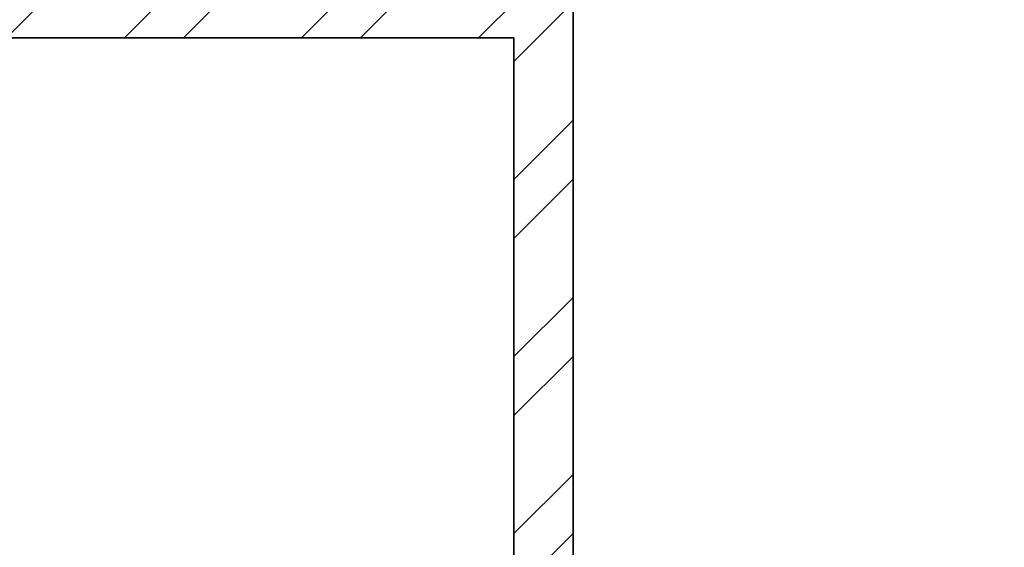
# Model space of a CAD drawing. Units: inches. Extents: x 1885 to 2748, y 783 to 2421.
# Tile 108 of 117: x 2449 to 2524, y 2027 to 2067. Entities that reach past the tile are written whole.
import ezdxf

# ---------------------------------------------------------------- set-up
doc = ezdxf.new("R2010")
doc.units = ezdxf.units.IN
doc.layers.add('A-WALL', color=7, linetype='Continuous', lineweight=35)
doc.layers.add('A-WALL-PATT', color=85, linetype='Continuous', lineweight=13, true_color=0x58ba48)

msp = doc.modelspace()

# ---------------------------------------------------------------- hatches: boundary and pattern name
at = {"layer": 'A-WALL-PATT'}
h = msp.add_hatch(dxfattribs=at)
h.set_pattern_fill('ANSI32', color=256)
h.paths.add_polyline_path([(2007.772, 2318.006), (1980.774, 2318.006), (1980.774, 2281.215), (1985.274, 2281.215), (1985.274, 2313.506), (2007.772, 2313.506), (2007.772, 2315.756)])
h.paths.add_polyline_path([(2094.324, 2318.006), (2067.772, 2318.006), (2067.772, 2313.506), (2094.324, 2313.506), (2094.324, 2315.756)])
h.paths.add_polyline_path([(2131.367, 2315.756), (2131.367, 2318.006), (2131.189, 2318.006), (2112.609, 2318.006), (2112.609, 2313.506), (2117.274, 2313.506), (2117.274, 2255.201), (2121.774, 2255.201), (2121.774, 2313.506), (2131.367, 2313.506)])
h.paths.add_polyline_path([(2190.512, 2318.006), (2155.367, 2318.006), (2155.367, 2313.506), (2169.774, 2313.506), (2169.774, 2229.506), (2121.774, 2229.506), (2121.774, 2233.451), (2119.524, 2233.451), (2117.274, 2233.451), (2117.274, 2201.101), (2121.774, 2201.101), (2121.774, 2225.006), (2169.774, 2225.006), (2169.774, 2165.006), (2306.274, 2165.006), (2306.274, 2066.006), (2310.774, 2066.006), (2344.274, 2066.006), (2486.274, 2066.006), (2486.274, 1886.006), (2483.02, 1886.006), (2483.02, 1881.506), (2486.274, 1881.506), (2486.274, 1880.678), (2490.774, 1880.678), (2490.774, 2070.506), (2344.274, 2070.506), (2310.774, 2070.506), (2310.774, 2165.006), (2310.774, 2173.636), (2308.524, 2173.636), (2306.274, 2173.636), (2306.274, 2169.506), (2174.274, 2169.506), (2174.274, 2313.506), (2190.512, 2313.506), (2190.512, 2315.756)])
h.paths.add_polyline_path([(1985.274, 2221.215), (1980.774, 2221.215), (1980.774, 2165.006), (1992.774, 2165.006), (1992.774, 2141.927), (1997.274, 2141.927), (1997.274, 2165.006), (2117.274, 2165.006), (2117.274, 2163.126), (2121.774, 2163.126), (2121.774, 2172.734), (2119.524, 2172.734), (2117.274, 2172.734), (2117.274, 2169.506), (1985.274, 2169.506)])
h.paths.add_polyline_path([(1997.274, 2105.927), (1992.774, 2105.927), (1992.774, 2070.506), (2016.774, 2070.506), (2016.774, 2059.123), (2019.024, 2059.123), (2021.274, 2059.123), (2021.274, 2070.506), (2117.274, 2070.506), (2117.274, 2022.506), (2114.423, 2022.506), (2114.423, 2018.006), (2123.627, 2018.006), (2123.627, 2020.256), (2123.627, 2022.506), (2121.774, 2022.506), (2121.774, 2142.587), (2119.524, 2142.587), (2117.274, 2142.587), (2117.274, 2075.006), (1997.274, 2075.006)])
h.paths.add_polyline_path([(2092.029, 2020.256), (2092.029, 2022.506), (2021.274, 2022.506), (2021.274, 2035.123), (2016.774, 2035.123), (2016.774, 2018.006), (2016.774, 1978.784), (2021.274, 1978.784), (2021.274, 2018.006), (2092.029, 2018.006)])
h.paths.add_polyline_path([(2260.938, 2022.506), (2153.105, 2022.506), (2153.105, 2020.256), (2153.105, 2018.006), (2155.274, 2018.006), (2155.274, 1886.006), (2107.629, 1886.006), (2107.629, 1881.506), (2182.911, 1881.506), (2182.911, 1883.756), (2182.911, 1886.006), (2159.774, 1886.006), (2159.774, 2018.006), (2260.938, 2018.006), (2260.938, 2020.256)])
h.paths.add_polyline_path([(2047.629, 1883.756), (2047.629, 1886.006), (2021.274, 1886.006), (2021.274, 1918.784), (2019.024, 1918.784), (2016.774, 1918.784), (2016.774, 1881.506), (2047.629, 1881.506)])
h.paths.add_polyline_path([(2306.361, 1883.756), (2306.361, 1886.006), (2296.274, 1886.006), (2296.274, 1982.006), (2316.535, 1982.006), (2316.535, 1984.256), (2316.535, 1986.506), (2296.274, 1986.506), (2296.274, 2022.506), (2289.276, 2022.506), (2289.276, 2018.006), (2291.774, 2018.006), (2291.774, 1886.006), (2242.911, 1886.006), (2242.911, 1881.506), (2306.361, 1881.506)], flags=17)
h.paths.add_polyline_path([(1985.274, 1843.006), (2021.6, 1843.006), (2021.534, 1845.441), (2021.477, 1847.506), (1980.774, 1847.506), (1980.774, 1809.446), (1985.274, 1809.446)])
h.paths.add_polyline_path([(2131.482, 1845.256), (2131.482, 1847.506), (2081.534, 1847.506), (2081.534, 1843.006), (2117.274, 1843.006), (2117.274, 1784.147), (2119.524, 1784.147), (2121.774, 1784.147), (2121.774, 1843.006), (2131.482, 1843.006)])
h.paths.add_polyline_path([(2203.886, 1847.506), (2155.482, 1847.506), (2155.482, 1843.006), (2169.774, 1843.006), (2169.774, 1759.006), (2121.774, 1759.006), (2121.774, 1761.457), (2117.274, 1761.457), (2117.274, 1730.429), (2121.774, 1730.429), (2121.774, 1754.506), (2177.421, 1754.506), (2177.421, 1756.756), (2177.421, 1759.006), (2174.274, 1759.006), (2174.274, 1843.006), (2203.886, 1843.006)])
h.paths.add_polyline_path([(2335.554, 1845.256), (2335.554, 1847.506), (2239.886, 1847.506), (2239.886, 1843.006), (2306.274, 1843.006), (2306.274, 1759.006), (2199.486, 1759.006), (2199.486, 1754.506), (2310.774, 1754.506), (2310.774, 1843.006), (2335.554, 1843.006)])
h.paths.add_polyline_path([(2348.774, 2022.506), (2344.274, 2022.506), (2344.274, 1986.506), (2341.681, 1986.506), (2341.681, 1982.006), (2344.274, 1982.006), (2344.274, 1886.006), (2330.361, 1886.006), (2330.361, 1881.506), (2361.627, 1881.506), (2361.627, 1883.756), (2361.627, 1886.006), (2348.774, 1886.006)], flags=17)
h.paths.add_polyline_path([(2283.251, 2315.756), (2283.251, 2318.006), (2238.512, 2318.006), (2238.512, 2313.506), (2283.251, 2313.506)], flags=17)
h.paths.add_polyline_path([(2363.274, 2348.006), (2388.677, 2348.006), (2388.677, 2350.256), (2388.677, 2352.506), (2358.774, 2352.506), (2358.774, 2348.006), (2358.774, 2318.006), (2344.481, 2318.006), (2344.481, 2313.506), (2358.774, 2313.506), (2358.774, 2229.506), (2310.774, 2229.506), (2310.774, 2231.952), (2306.274, 2231.952), (2306.274, 2205.611), (2310.774, 2205.611), (2310.774, 2225.006), (2358.774, 2225.006), (2358.774, 2211.506), (2452.329, 2211.506), (2452.329, 2213.756), (2452.329, 2216.006), (2363.274, 2216.006), (2363.274, 2318.006)])
h.paths.add_polyline_path([(2310.774, 2313.506), (2320.481, 2313.506), (2320.481, 2315.756), (2320.481, 2318.006), (2302.728, 2318.006), (2302.728, 2313.506), (2306.274, 2313.506), (2306.274, 2251.076), (2310.774, 2251.076)], flags=17)
h.paths.add_polyline_path([(2490.774, 2352.506), (2486.274, 2352.506), (2448.677, 2352.506), (2448.677, 2348.006), (2486.274, 2348.006), (2486.274, 2318.006), (2486.274, 2216.006), (2481.78, 2216.006), (2481.78, 2211.506), (2486.274, 2211.506), (2486.274, 2165.006), (2493.289, 2165.006), (2493.289, 2167.256), (2493.289, 2169.506), (2490.774, 2169.506), (2490.774, 2313.506), (2494.429, 2313.506), (2494.429, 2318.006), (2490.774, 2318.006)])
h.paths.add_polyline_path([(2534.653, 2318.006), (2515.691, 2318.006), (2515.691, 2313.506), (2534.653, 2313.506), (2534.653, 2315.756)])
h.paths.add_polyline_path([(2618.274, 2318.006), (2594.653, 2318.006), (2594.653, 2313.506), (2613.774, 2313.506), (2613.774, 2281.706), (2618.274, 2281.706)])
h.paths.add_polyline_path([(2618.274, 2221.706), (2613.774, 2221.706), (2613.774, 2169.506), (2554.019, 2169.506), (2554.019, 2165.006), (2613.774, 2165.006), (2613.774, 2152.878), (2618.274, 2152.878)])
h.paths.add_polyline_path([(2618.274, 2128.878), (2616.024, 2128.878), (2613.774, 2128.878), (2613.774, 2117.006), (2529.774, 2117.006), (2529.774, 2165.006), (2532.848, 2165.006), (2532.848, 2169.506), (2522.867, 2169.506), (2522.867, 2165.006), (2525.274, 2165.006), (2525.274, 2117.006), (2525.274, 2112.506), (2525.274, 2108.576), (2529.774, 2108.576), (2529.774, 2112.506), (2613.774, 2112.506), (2613.774, 2080.19), (2618.274, 2080.19)])
h.paths.add_polyline_path([(2618.274, 2044.19), (2616.024, 2044.19), (2613.774, 2044.19), (2613.774, 2015.506), (2529.774, 2015.506), (2529.774, 2088.582), (2527.524, 2088.582), (2525.274, 2088.582), (2525.274, 2011.006), (2613.774, 2011.006), (2613.774, 1956.755), (2618.274, 1956.755)])
h.paths.add_polyline_path([(2618.274, 1881.506), (2618.274, 1896.755), (2613.774, 1896.755), (2613.774, 1881.506), (2613.774, 1847.506), (2592.715, 1847.506), (2592.715, 1843.006), (2613.774, 1843.006), (2613.774, 1765.006), (2613.774, 1760.506), (2609.621, 1760.506), (2609.621, 1756.006), (2613.774, 1756.006), (2613.774, 1660.006), (2608.544, 1660.006), (2608.544, 1655.506), (2613.774, 1655.506), (2613.774, 1508.158), (2618.274, 1508.158)])
h.paths.add_polyline_path([(2565.774, 1843.006), (2568.997, 1843.006), (2568.997, 1847.506), (2490.774, 1847.506), (2490.774, 1849.7), (2488.524, 1849.7), (2486.274, 1849.7), (2486.274, 1847.506), (2477.274, 1847.506), (2477.274, 1838.506), (2477.274, 1821.493), (2486.274, 1821.493), (2486.274, 1838.506), (2561.274, 1838.506), (2561.274, 1765.006), (2486.274, 1765.006), (2486.274, 1786.157), (2477.274, 1786.157), (2477.274, 1765.006), (2477.274, 1756.006), (2486.274, 1756.006), (2565.774, 1756.006), (2585.621, 1756.006), (2585.621, 1758.256), (2585.621, 1760.506), (2565.774, 1760.506), (2565.774, 1765.006)])
h.paths.add_polyline_path([(2486.274, 1651.006), (2561.274, 1651.006), (2561.274, 1567.006), (2486.274, 1567.006), (2486.274, 1591.321), (2477.274, 1591.321), (2477.274, 1567.006), (2477.274, 1558.006), (2477.274, 1555.439), (2481.774, 1555.439), (2481.774, 1558.006), (2568.653, 1558.006), (2568.653, 1560.256), (2568.653, 1562.506), (2565.774, 1562.506), (2565.774, 1655.506), (2584.544, 1655.506), (2584.544, 1657.756), (2584.544, 1660.006), (2565.774, 1660.006), (2486.274, 1660.006), (2477.274, 1660.006), (2477.274, 1651.006), (2477.274, 1632.989), (2486.274, 1632.989)])
h.paths.add_polyline_path([(2449.967, 1883.756), (2449.967, 1886.006), (2421.627, 1886.006), (2421.627, 1881.506), (2449.967, 1881.506)], flags=17)
h.paths.add_polyline_path([(2447.274, 1847.506), (2395.554, 1847.506), (2395.554, 1843.006), (2442.774, 1843.006), (2442.774, 1809.27), (2447.274, 1809.27)])
h.paths.add_polyline_path([(1985.274, 1749.446), (1980.774, 1749.446), (1980.774, 1694.504), (1985.274, 1694.504), (1985.274, 1694.506), (1986.897, 1694.506), (1986.897, 1697.78), (1986.897, 1699.006), (1985.274, 1699.006)])
h.paths.add_polyline_path([(2152.774, 1699.006), (2121.774, 1699.006), (2121.774, 1703.668), (2119.524, 1703.668), (2117.274, 1703.668), (2117.274, 1699.006), (2009.219, 1699.006), (2009.219, 1694.506), (2148.274, 1694.506), (2148.274, 1692.631), (2152.774, 1692.631)])
h.paths.add_polyline_path([(2016.274, 1694.506), (2011.774, 1694.506), (2011.774, 1558.006), (2040.806, 1558.006), (2040.806, 1560.256), (2040.806, 1562.506), (2016.274, 1562.506)])
h.paths.add_polyline_path([(2152.774, 1663.017), (2150.524, 1663.017), (2148.274, 1663.017), (2148.274, 1562.506), (2100.806, 1562.506), (2100.806, 1558.006), (2165.119, 1558.006), (2165.119, 1560.256), (2165.119, 1562.506), (2152.774, 1562.506), (2152.774, 1610.506), (2224.774, 1610.506), (2224.774, 1607.99), (2229.274, 1607.99), (2229.274, 1615.006), (2152.774, 1615.006)])
h.paths.add_polyline_path([(2238.613, 1560.256), (2238.613, 1562.506), (2229.274, 1562.506), (2229.274, 1588.756), (2227.024, 1588.763), (2224.774, 1588.771), (2224.774, 1562.506), (2189.119, 1562.506), (2189.119, 1558.006), (2238.613, 1558.006)])
h.paths.add_polyline_path([(2336.024, 1560.256), (2336.024, 1562.506), (2310.774, 1562.506), (2310.774, 1656.347), (2308.524, 1656.347), (2306.274, 1656.347), (2306.274, 1562.506), (2286.613, 1562.506), (2286.613, 1558.006), (2336.024, 1558.006)])
h.paths.add_polyline_path([(2447.274, 1690.968), (2445.024, 1690.968), (2442.774, 1690.968), (2442.774, 1687.006), (2306.274, 1687.006), (2306.274, 1680.75), (2310.774, 1680.75), (2310.774, 1682.506), (2442.774, 1682.506), (2442.774, 1562.506), (2396.024, 1562.506), (2396.024, 1558.006), (2447.274, 1558.006)])
h.paths.add_polyline_path([(2447.274, 1749.27), (2445.024, 1749.27), (2442.774, 1749.27), (2442.774, 1717.232), (2447.274, 1717.232)])
h.paths.add_polyline_path([(2044.674, 1521.756), (2044.674, 1524.006), (2007.274, 1524.006), (2007.274, 1503.49), (2009.524, 1503.49), (2011.774, 1503.49), (2011.774, 1519.506), (2044.674, 1519.506)])
h.paths.add_polyline_path([(2177.969, 1521.756), (2177.969, 1524.006), (2104.674, 1524.006), (2104.674, 1519.506), (2145.774, 1519.506), (2145.774, 1387.506), (2143.37, 1387.506), (2143.37, 1383.006), (2251.585, 1383.006), (2251.585, 1385.256), (2251.585, 1387.506), (2150.274, 1387.506), (2150.274, 1519.506), (2177.969, 1519.506)])
h.paths.add_polyline_path([(2298.704, 1524.006), (2237.969, 1524.006), (2237.969, 1519.506), (2282.274, 1519.506), (2282.274, 1387.506), (2279.683, 1387.506), (2279.683, 1383.006), (2286.774, 1383.006), (2286.774, 1419.006), (2312.451, 1419.006), (2312.451, 1421.256), (2312.451, 1423.506), (2286.774, 1423.506), (2286.774, 1519.506), (2298.704, 1519.506), (2298.704, 1521.722)], flags=17)
h.paths.add_polyline_path([(2361.897, 1521.756), (2361.897, 1524.006), (2322.704, 1524.006), (2322.704, 1519.506), (2334.774, 1519.506), (2334.774, 1423.506), (2331.93, 1423.506), (2331.93, 1419.006), (2334.774, 1419.006), (2334.774, 1387.506), (2334.774, 1383.228), (2339.274, 1383.228), (2339.274, 1387.506), (2339.274, 1519.506), (2361.897, 1519.506)], flags=17)
h.paths.add_polyline_path([(2447.274, 1521.756), (2447.274, 1524.006), (2421.897, 1524.006), (2421.897, 1519.506), (2447.274, 1519.506)], flags=17)
h.paths.add_polyline_path([(2481.774, 1529.6), (2479.524, 1529.6), (2477.274, 1529.6), (2477.274, 1524.006), (2474.489, 1524.006), (2474.489, 1519.506), (2477.274, 1519.506), (2477.274, 1334.506), (2296.774, 1334.506), (2296.774, 1240.506), (2160.274, 1240.506), (2160.274, 1180.506), (2112.274, 1180.506), (2112.274, 1207.692), (2110.024, 1207.692), (2107.774, 1207.692), (2107.774, 1171.609), (2112.274, 1171.609), (2112.274, 1176.006), (2160.274, 1176.006), (2160.274, 1092.006), (2144.221, 1092.006), (2144.221, 1087.506), (2189.497, 1087.506), (2189.497, 1089.756), (2189.497, 1092.006), (2164.774, 1092.006), (2164.774, 1236.006), (2296.774, 1236.006), (2296.774, 1231.912), (2301.274, 1231.912), (2301.274, 1330.006), (2481.774, 1330.006), (2481.774, 1387.506)])
h.paths.add_polyline_path([(2618.274, 1448.158), (2613.774, 1448.158), (2613.774, 1382.506), (2529.774, 1382.506), (2525.274, 1382.506), (2525.274, 1307.062), (2529.774, 1307.062), (2529.774, 1378.006), (2613.774, 1378.006), (2613.774, 1354.988), (2618.274, 1354.988)])
h.paths.add_polyline_path([(2618.274, 1318.988), (2613.774, 1318.988), (2613.774, 1281.006), (2529.774, 1281.006), (2529.774, 1283.786), (2527.524, 1283.786), (2525.274, 1283.786), (2525.274, 1228.506), (2516.794, 1228.506), (2516.794, 1224.006), (2533.484, 1224.006), (2533.484, 1226.256), (2533.484, 1228.506), (2529.774, 1228.506), (2529.774, 1276.506), (2613.774, 1276.506), (2613.774, 1266.02), (2618.274, 1266.02)])
h.paths.add_polyline_path([(2618.274, 1134.964), (2613.774, 1134.964), (2613.774, 1092.006), (2594.545, 1092.006), (2594.545, 1087.506), (2618.274, 1087.506)])
h.paths.add_polyline_path([(2534.545, 1092.006), (2509.765, 1092.006), (2509.765, 1087.506), (2534.545, 1087.506), (2534.545, 1089.756)])
h.paths.add_polyline_path([(2481.274, 1224.006), (2484.117, 1224.006), (2484.117, 1226.256), (2484.117, 1228.506), (2476.774, 1228.506), (2476.774, 1198.506), (2471.61, 1198.506), (2471.61, 1194.006), (2476.774, 1194.006), (2476.774, 1062.006), (2436.894, 1062.006), (2436.894, 1057.506), (2476.774, 1057.506), (2481.274, 1057.506), (2481.274, 1062.006), (2481.274, 1087.506), (2485.354, 1087.506), (2485.354, 1089.756), (2485.354, 1092.006), (2481.274, 1092.006), (2481.274, 1117.506)])
h.paths.add_polyline_path([(2439.898, 1198.506), (2349.274, 1198.506), (2349.274, 1194.006), (2349.274, 1180.506), (2301.274, 1180.506), (2301.274, 1201.896), (2299.024, 1201.896), (2296.774, 1201.896), (2296.774, 1172.335), (2299.024, 1172.335), (2301.274, 1172.335), (2301.274, 1176.006), (2349.274, 1176.006), (2349.274, 1092.006), (2334.452, 1092.006), (2334.452, 1087.506), (2349.274, 1087.506), (2349.274, 1057.506), (2353.774, 1057.506), (2376.894, 1057.506), (2376.894, 1059.756), (2376.894, 1062.006), (2353.774, 1062.006), (2353.774, 1087.506), (2353.774, 1180.506), (2353.774, 1194.006), (2439.898, 1194.006), (2439.898, 1196.256)])
h.paths.add_polyline_path([(2270.596, 1089.756), (2270.596, 1092.006), (2249.497, 1092.006), (2249.497, 1087.506), (2270.596, 1087.506)], flags=17)
h.paths.add_polyline_path([(2310.452, 1092.006), (2301.274, 1092.006), (2301.274, 1153.292), (2296.774, 1153.292), (2296.774, 1092.006), (2293.786, 1092.006), (2293.786, 1087.506), (2310.452, 1087.506), (2310.452, 1089.756)], flags=17)
h.paths.add_polyline_path([(2112.274, 1150.328), (2110.024, 1150.328), (2107.774, 1150.328), (2107.774, 1092.006), (2104.465, 1092.006), (2104.465, 1087.506), (2120.221, 1087.506), (2120.221, 1089.756), (2120.221, 1092.006), (2112.274, 1092.006)])
h.paths.add_polyline_path([(2082.172, 1092.006), (2058.144, 1092.006), (2058.144, 1087.506), (2082.172, 1087.506), (2082.172, 1089.756)])
h.paths.add_polyline_path([(1975.774, 1145.638), (1971.274, 1145.638), (1971.274, 1087.506), (1980.774, 1087.506), (1998.144, 1087.506), (1998.144, 1089.756), (1998.144, 1092.006), (1985.274, 1092.006), (1975.774, 1092.006)])
h.paths.add_polyline_path([(2112.274, 1244.385), (2110.024, 1244.385), (2107.774, 1244.385), (2107.774, 1240.506), (1992.274, 1240.506), (1992.274, 1271.008), (1987.774, 1271.008), (1987.774, 1240.506), (1980.774, 1240.506), (1975.774, 1240.506), (1971.274, 1240.506), (1971.274, 1205.638), (1975.774, 1205.638), (1975.774, 1236.006), (2107.774, 1236.006), (2107.774, 1233.444), (2112.274, 1233.444), (2112.274, 1236.006)])
h.paths.add_polyline_path([(2112.274, 1383.006), (2114.783, 1383.006), (2114.783, 1385.256), (2114.783, 1387.506), (2102.476, 1387.506), (2102.476, 1383.006), (2107.774, 1383.006), (2107.774, 1335.006), (2011.774, 1335.006), (2011.774, 1349.939), (2007.274, 1349.939), (2007.274, 1335.006), (1987.774, 1335.006), (1987.774, 1330.506), (1987.774, 1307.008), (1992.274, 1307.008), (1992.274, 1330.506), (2007.274, 1330.506), (2107.774, 1330.506), (2107.774, 1264.711), (2112.274, 1264.711)])
h.paths.add_polyline_path([(2077.857, 1387.506), (2011.774, 1387.506), (2011.774, 1390.036), (2009.524, 1390.036), (2007.274, 1390.036), (2007.274, 1373.939), (2011.774, 1373.939), (2011.774, 1383.006), (2077.857, 1383.006)])
h.paths.add_polyline_path([(2011.774, 1443.49), (2007.274, 1443.49), (2007.274, 1410.248), (2011.774, 1410.248)])

# ---------------------------------------------------------------- linework, layer by layer
at = {"layer": 'A-WALL'}
for p, q in [((2490.774, 2070.506), (2490.774, 1879.236)), ((2486.274, 2066.006), (2344.274, 2066.006)), ((2486.274, 2066.006), (2486.274, 1886.006))]:
    msp.add_line(p, q, dxfattribs=at)

doc.saveas('drawing.dxf')
